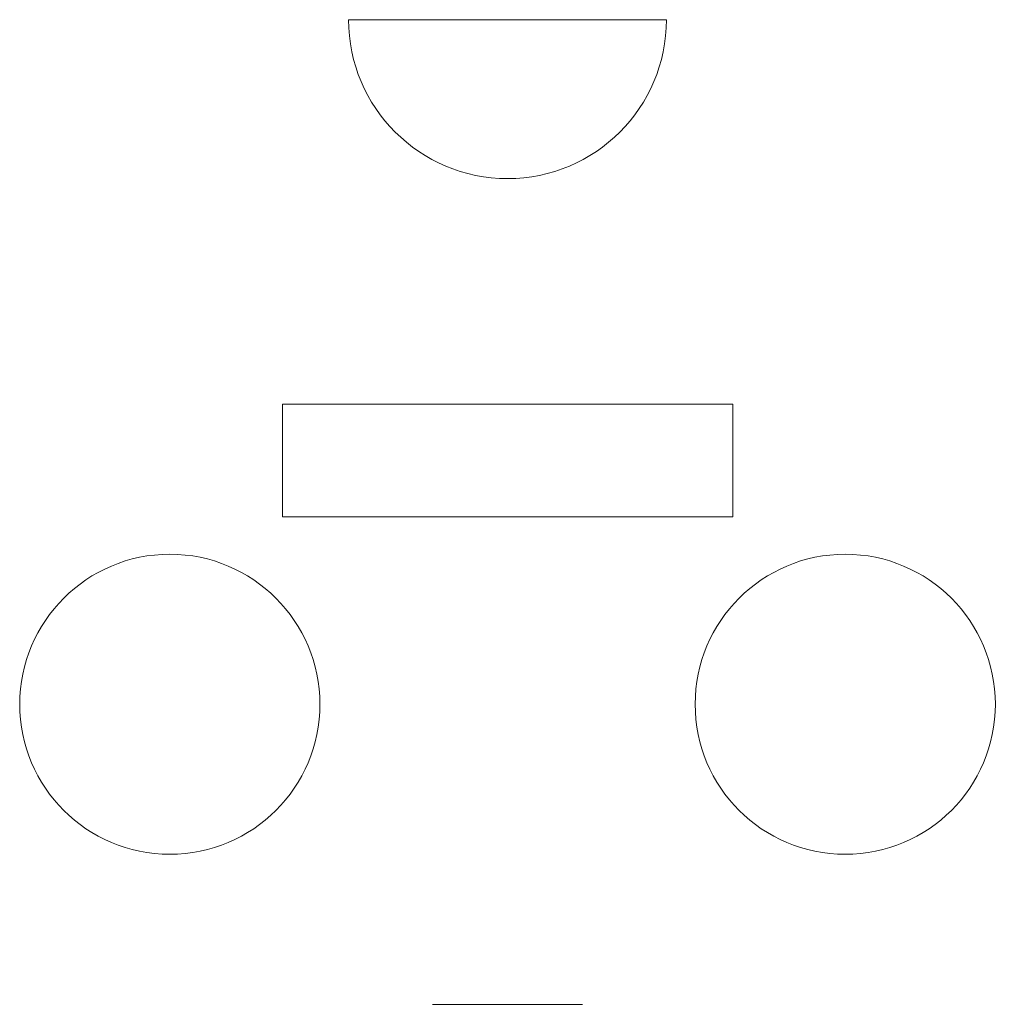
# Model space of a CAD drawing. Units: inches. Extents: x -235 to -131, y 69 to 174.
import ezdxf

# ---------------------------------------------------------------- set-up
doc = ezdxf.new("R2010")
doc.units = ezdxf.units.IN
doc.header["$MEASUREMENT"] = 0
doc.layers.add('M-CONS', color=8, linetype='Continuous', lineweight=13)

msp = doc.modelspace()

# ---------------------------------------------------------------- linework, layer by layer
at = {"layer": 'M-CONS'}
for p, q in [((-166.52, 174.45, 19), (-200.4, 174.45, 19)), ((-200.4, 174.45, 19), (-166.52, 174.45, 19)), ((-183.46, 69.45), (-191.46, 69.45))]:
    msp.add_line(p, q, dxfattribs=at)
at = {"layer": 'M-CONS', "extrusion": (0, 0, -1)}
for p, q in [((-207.46, 121.45), (-207.46, 133.45)), ((-159.46, 133.45), (-207.46, 133.45)), ((-207.46, 133.45), (-159.46, 133.45)), ((-159.46, 121.45), (-159.46, 133.45)), ((-183.46, 121.45), (-207.46, 121.45)), ((-183.46, 121.45), (-159.46, 121.45)), ((-183.46, 69.45), (-175.46, 69.45))]:
    msp.add_line(p, q, dxfattribs=at)
at = {"layer": 'M-CONS', "elevation": 42.44}
msp.add_lwpolyline([(-200.4, 174.45, 1), (-166.52, 174.45)], format="xyb", close=True, dxfattribs=at)
at = {"layer": 'M-CONS'}
for centre in [(-219.46, 101.45), (-147.46, 101.45)]:
    msp.add_circle(centre, 16, dxfattribs=at)
msp.add_arc((-183.46, 174.45, 19), 16.94, 180, 0, dxfattribs=at)

doc.saveas('drawing.dxf')
